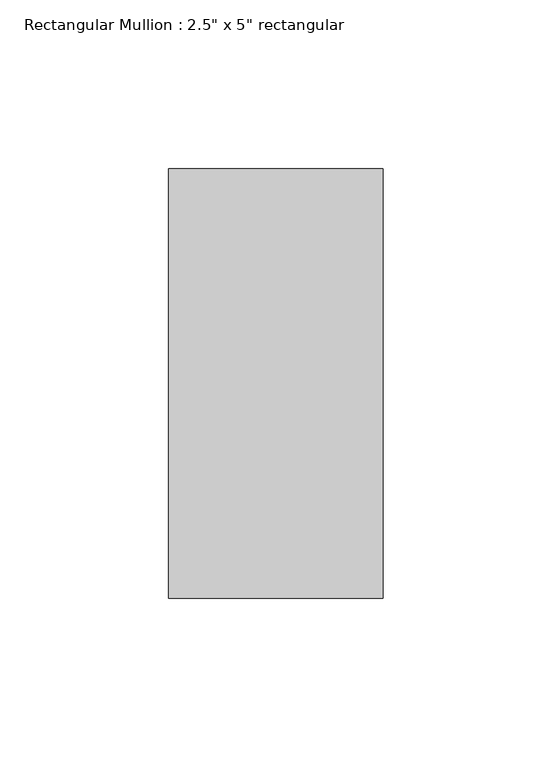
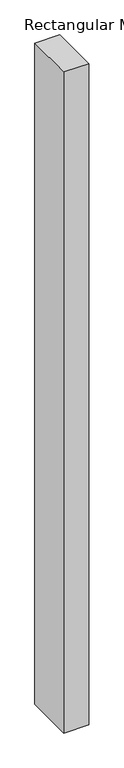
"""IFC4 building model written with IfcOpenShell, lengths in millimetres: member geometry."""

from ifc_helpers import new_model, si_unit, frame, origin, place, context, project, spatial, polyline, outline, extrude, source, transform, mapped, element, save


def member_ec261fe8(model_context):
    return source(origin(), model_context, "Body", "SweptSolid", [
        extrude(outline(polyline([(31.75, 63.5), (31.75, -63.5), (-31.75, -63.5), (-31.75, 63.5), (31.75, 63.5)])), frame((0.0, 0.0, -1778.0), z_axis=(0.0, 0.0, 1.0), x_axis=(1.0, 0.0, 0.0)), (0.0, 0.0, 1.0), 1778.0),
    ])


if __name__ == "__main__":
    model = new_model("IFC4")
    model_context = context("Model", 3, world=origin())
    ifc_project = project(units=[si_unit("LENGTHUNIT", "METRE", prefix="MILLI")], contexts=[model_context])
    site = spatial("IfcSite", under=ifc_project)
    building = spatial("IfcBuilding", under=site)
    placement = place(None, origin())
    member_shape = member_ec261fe8(model_context)
    element("IfcMember", 1, ObjectType="Rectangular Mullion : 2.5\" x 5\" rectangular", at=placement, inside=building, context=model_context, shape_type="MappedRepresentation", body=[
        mapped(member_shape, transform((0.0, 0.0, 0.0), x_axis=(1.0, 0.0, 0.0), y_axis=(0.0, 1.0, 0.0), z_axis=(0.0, 0.0, 1.0))),
    ])
    save(model, "model.ifc")

# Revit data of these elements
# Type "Rectangular Mullion : 2.5\" x 5\" rectangular"
#   built-in parameter 1007304 = 0.416667 (stored number, unit not read)
#   built-in parameter 1007301 = 0.104167 (stored number, unit not read)
#   built-in parameter 1007300 = 0.104167 (stored number, unit not read)
# Element 1 (IfcMember, "Rectangular Mullion : 2.5\" x 5\" rectangular")
#   Materials on its faces: "Aluminum"
# Materials
#   "Aluminum": class "Metal", colour RGB 247 247 247, transparency 0, Description = "Aluminum 6061", Cost = 0
